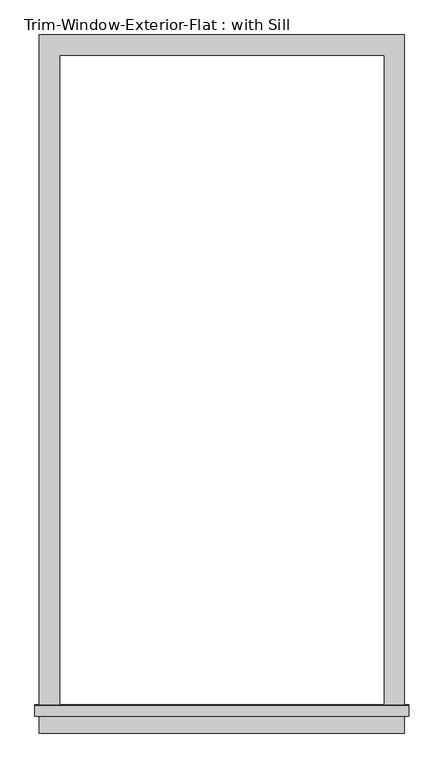
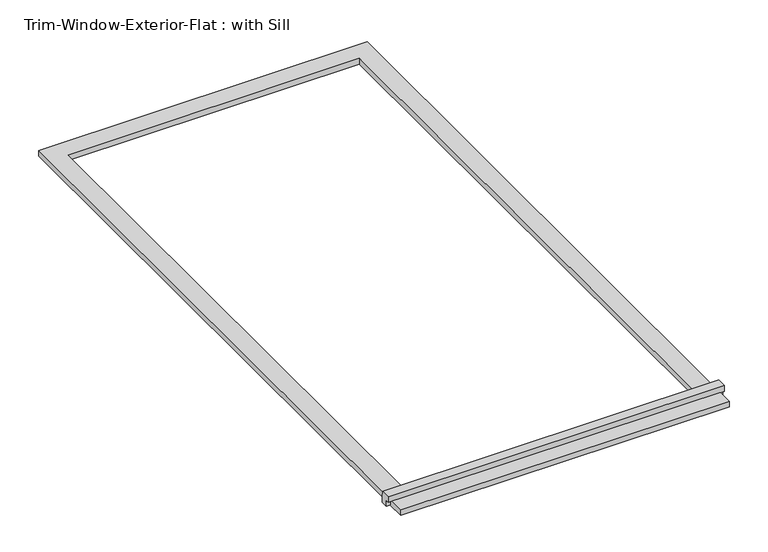
"""IFC4 building model written with IfcOpenShell, lengths in millimetres: proxy geometry, Trim-Window-Exterior-Flat : with Sill."""

from ifc_helpers import new_model, si_unit, frame, origin, origin_with_axes, place, context, project, spatial, polyline, outline, extrude, source, transform, mapped, element, save


def trim_window_exterior_flat_with_sill_c2ca58d6(model_context):
    return source(origin(), model_context, "Body", "SweptSolid", [
        extrude(outline(polyline([(514.35, -1850.9823709), (514.35, -1908.1323709), (-514.35, -1908.1323709), (-514.35, -1850.9823709), (514.35, -1850.9823709)])), origin_with_axes(), (0.0, 0.0, 1.0), 19.05),
        extrude(outline(polyline([(-1860.55, 38.1), (-1831.2580645, 38.1), (-1828.8, 19.05), (-1828.8, 0.0), (-1850.9823709, 0.0), (-1850.9823709, 19.05), (-1860.55, 19.05), (-1860.55, 38.1)])), frame((-527.05, 0.0, 0.0), z_axis=(1.0, 0.0, 0.0), x_axis=(0.0, 1.0, 0.0)), (0.0, 0.0, 1.0), 1054.1),
        extrude(outline(polyline([(-514.35, 57.15), (514.35, 57.15), (514.35, -1828.8), (457.2, -1828.8), (457.2, 0.0), (-457.2, 0.0), (-457.2, -1828.8), (-514.35, -1828.8), (-514.35, 57.15)])), origin_with_axes(), (0.0, 0.0, 1.0), 19.05),
    ])


if __name__ == "__main__":
    model = new_model("IFC4")
    model_context = context("Model", 3, world=origin())
    ifc_project = project(units=[si_unit("LENGTHUNIT", "METRE", prefix="MILLI")], contexts=[model_context])
    site = spatial("IfcSite", under=ifc_project)
    building = spatial("IfcBuilding", under=site)
    placement = place(None, origin())
    trim_window_exterior_flat_with_sill_shape = trim_window_exterior_flat_with_sill_c2ca58d6(model_context)
    element("IfcBuildingElementProxy", 1, Name="Trim-Window-Exterior-Flat : with Sill", ObjectType="Trim-Window-Exterior-Flat : with Sill", at=placement, inside=building, context=model_context, shape_type="MappedRepresentation", body=[
        mapped(trim_window_exterior_flat_with_sill_shape, transform((0.0, 0.0, 0.0), x_axis=(1.0, 0.0, 0.0), y_axis=(0.0, 1.0, 0.0), z_axis=(0.0, 0.0, 1.0))),
    ])
    save(model, "model.ifc")

# Revit data of these elements
# Type "Trim-Window-Exterior-Flat : with Sill"
#   Trim Width = 0' - 2 1/4"
#   Trim Thickness_Picture Frame = 0' - 1 1/4"
#   Trim Thickness_with Sill = 0' - 0 3/4"
#   Sill Thickness = 0' - 1 1/4"
#   Opening Width [instance default] = 2' - 0"
#   Opening Height [instance default] = 3' - 0"
#   Default Elevation = 4' - 0"
#   Sill = yes
#   Picture Frame = no
#   Trim Material [instance default] = none
# Element 1 (IfcBuildingElementProxy, "Trim-Window-Exterior-Flat : with Sill")
#   Opening Width = 3' - 0"
#   Opening Height = 6' - 0"
#   Trim Material = Clad - White
#   Materials on its faces: "Clad - White"
# Materials
#   "Clad - White": class "Wood", colour RGB 242 242 238, transparency 0, Cost = 0
